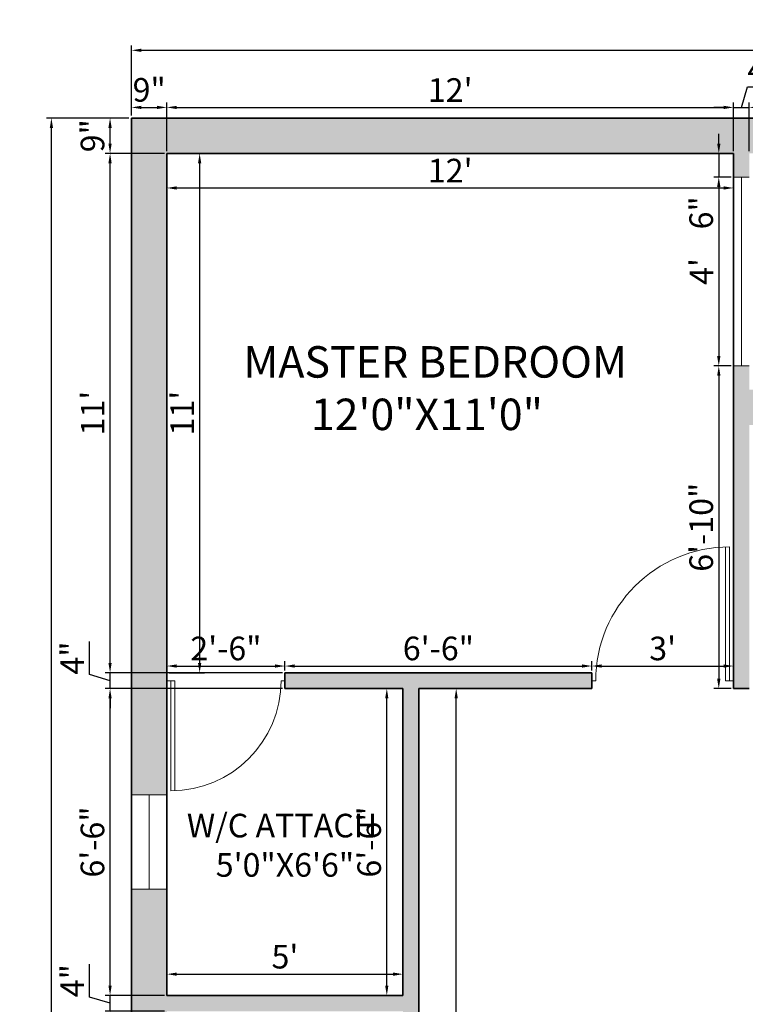
# Model space of a CAD drawing. Units: inches. Extents: x 3592 to 4861, y 1650 to 2243.
# Tile 29 of 30: x 4438 to 4622, y 1940 to 2190. Entities that reach past the tile are written whole.
import ezdxf

# ---------------------------------------------------------------- set-up
doc = ezdxf.new("R2010")
doc.units = ezdxf.units.IN
for name, color, linetype, lineweight in [('A-ANNO-DIMS', 2, 'Continuous', 13), ('A-AREA-IDEN', 7, 'Continuous', 18), ('A-DOOR', 3, 'Continuous', 20), ('A-GLAZ', 4, 'Continuous', 18), ('A-WALL', 7, 'Continuous', 35)]:
    doc.layers.add(name, color=color, linetype=linetype, lineweight=lineweight)
doc.layers.add('A-WALL-PATT', color=252, linetype='Continuous', lineweight=13, true_color=0x939598)
doc.styles.get("Standard").update_dxf_attribs({"font": 'arial.ttf'})
doc.dimstyles.new('ISO-25', dxfattribs={"dimtxt": 9, "dimasz": 2.5, "dimexe": 1.25, "dimexo": 0.625, "dimtad": 1, "dimlunit": 3, "dimtxsty": 'Standard', "dimcen": 2.5, "dimadec": 0, "dimazin": 0, "dimtfac": 1, "dimtmove": 0, "dimatfit": 3, "dimfxl": 1, "dimarcsym": 0})

# ---------------------------------------------------------------- blocks, each defined once
blk = doc.blocks.new('1')
for p, q in [((3628.27, 1890.86), (3628.27, 1924.86)), ((3629.27, 1890.86), (3629.27, 1924.86)), ((3627.27, 1890.86), (3629.27, 1890.86)), ((3662.27, 1890.86), (3663.27, 1890.86))]:
    blk.add_line(p, q)
blk.add_arc((3628.27, 1890.86), 34, 0, 90)
blk = doc.blocks.new('2')
for p, q in [((3637.19, 1914.49), (3637.19, 1942.49)), ((3638.19, 1914.49), (3638.19, 1942.49)), ((3636.19, 1914.49), (3638.19, 1914.49)), ((3665.19, 1914.49), (3666.19, 1914.49))]:
    blk.add_line(p, q)
blk.add_arc((3637.19, 1914.49), 28, 0, 90)
blk = doc.blocks.new('*D45')
at = {"layer": 'A-ANNO-DIMS', "color": 0, "lineweight": -2, "transparency": 16777216}
for p, q in [((4475.25, 2155.59), (4475.25, 2146.2)), ((4619.25, 2155.59), (4619.25, 2146.2)), ((4477.75, 2147.45), (4616.75, 2147.45))]:
    blk.add_line(p, q, dxfattribs=at)
at = {"layer": 'A-ANNO-DIMS', "color": 0, "transparency": 16777216}
for points in [[(4477.75, 2147.86), (4477.75, 2147.03), (4475.25, 2147.45)], [(4616.75, 2147.86), (4616.75, 2147.03), (4619.25, 2147.45)]]:
    blk.add_solid(points, dxfattribs=at)
at = {"layer": 'Defpoints', "color": 0, "transparency": 16777216}
for p in [(4475.25, 2156.22), (4619.25, 2156.22), (4619.25, 2147.45)]:
    blk.add_point(p, dxfattribs=at)
at = {"layer": 'A-ANNO-DIMS', "color": 0, "transparency": 16777216, "insert": (4547.25, 2151.08), "char_height": 6, "attachment_point": 5}
blk.add_mtext("12'", dxfattribs=at)
blk = doc.blocks.new('*D46')
at = {"layer": 'A-ANNO-DIMS', "color": 0, "lineweight": -2, "transparency": 16777216}
for p, q in [((4475.25, 2024.79), (4475.25, 2027.19)), ((4505.25, 2024.84), (4505.25, 2027.19)), ((4477.75, 2025.94), (4502.75, 2025.94))]:
    blk.add_line(p, q, dxfattribs=at)
at = {"layer": 'A-ANNO-DIMS', "color": 0, "transparency": 16777216}
for points in [[(4477.75, 2026.36), (4477.75, 2025.53), (4475.25, 2025.94)], [(4502.75, 2026.36), (4502.75, 2025.53), (4505.25, 2025.94)]]:
    blk.add_solid(points, dxfattribs=at)
at = {"layer": 'Defpoints', "color": 0, "transparency": 16777216}
for p in [(4505.25, 2025.94), (4475.25, 2024.17), (4505.25, 2024.22)]:
    blk.add_point(p, dxfattribs=at)
at = {"layer": 'A-ANNO-DIMS', "color": 0, "transparency": 16777216, "insert": (4490.25, 2029.63), "char_height": 6, "attachment_point": 5}
blk.add_mtext('2\'-6"', dxfattribs=at)
blk = doc.blocks.new('*D47')
at = {"layer": 'A-ANNO-DIMS', "color": 0, "lineweight": -2, "transparency": 16777216}
for p, q in [((4505.25, 2024.84), (4505.25, 2027.19)), ((4583.25, 2024.84), (4583.25, 2027.19)), ((4507.75, 2025.94), (4580.75, 2025.94))]:
    blk.add_line(p, q, dxfattribs=at)
at = {"layer": 'A-ANNO-DIMS', "color": 0, "transparency": 16777216}
for points in [[(4507.75, 2026.36), (4507.75, 2025.53), (4505.25, 2025.94)], [(4580.75, 2026.36), (4580.75, 2025.53), (4583.25, 2025.94)]]:
    blk.add_solid(points, dxfattribs=at)
at = {"layer": 'Defpoints', "color": 0, "transparency": 16777216}
for p in [(4583.25, 2025.94), (4505.25, 2024.22), (4583.25, 2024.22)]:
    blk.add_point(p, dxfattribs=at)
at = {"layer": 'A-ANNO-DIMS', "color": 0, "transparency": 16777216, "insert": (4544.25, 2029.63), "char_height": 6, "attachment_point": 5}
blk.add_mtext('6\'-6"', dxfattribs=at)
blk = doc.blocks.new('*D48')
at = {"layer": 'A-ANNO-DIMS', "color": 0, "lineweight": -2, "transparency": 16777216}
for p, q in [((4583.25, 2024.84), (4583.25, 2027.19)), ((4585.75, 2025.94), (4616.75, 2025.94)), ((4619.25, 2025.32), (4619.25, 2024.69))]:
    blk.add_line(p, q, dxfattribs=at)
at = {"layer": 'A-ANNO-DIMS', "color": 0, "transparency": 16777216}
for points in [[(4585.75, 2026.36), (4585.75, 2025.53), (4583.25, 2025.94)], [(4616.75, 2026.36), (4616.75, 2025.53), (4619.25, 2025.94)]]:
    blk.add_solid(points, dxfattribs=at)
at = {"layer": 'Defpoints', "color": 0, "transparency": 16777216}
for p in [(4619.25, 2025.94), (4619.25, 2025.94), (4583.25, 2024.22)]:
    blk.add_point(p, dxfattribs=at)
at = {"layer": 'A-ANNO-DIMS', "color": 0, "transparency": 16777216, "insert": (4601.25, 2029.63), "char_height": 6, "attachment_point": 5}
blk.add_mtext("3'", dxfattribs=at)
blk = doc.blocks.new('*D49')
at = {"layer": 'A-ANNO-DIMS', "color": 0, "lineweight": -2, "transparency": 16777216}
for p, q in [((4475.87, 2156.22), (4484.83, 2156.22)), ((4483.58, 2153.72), (4483.58, 2026.72)), ((4475.87, 2024.22), (4484.83, 2024.22))]:
    blk.add_line(p, q, dxfattribs=at)
at = {"layer": 'A-ANNO-DIMS', "color": 0, "transparency": 16777216}
for points in [[(4483.16, 2153.72), (4483.99, 2153.72), (4483.58, 2156.22)], [(4483.16, 2026.72), (4483.99, 2026.72), (4483.58, 2024.22)]]:
    blk.add_solid(points, dxfattribs=at)
at = {"layer": 'Defpoints', "color": 0, "transparency": 16777216}
for p in [(4475.25, 2156.22), (4475.25, 2024.22), (4483.58, 2024.22)]:
    blk.add_point(p, dxfattribs=at)
at = {"layer": 'A-ANNO-DIMS', "color": 0, "transparency": 16777216, "insert": (4479.94, 2090.22), "char_height": 6, "attachment_point": 5, "rotation": 90}
blk.add_mtext("11'", dxfattribs=at)
blk = doc.blocks.new('*D56')
at = {"layer": 'A-ANNO-DIMS', "color": 0, "lineweight": -2, "transparency": 16777216}
for p, q in [((4615.51, 2158.72), (4615.51, 2161.22)), ((4618.62, 2156.22), (4614.26, 2156.22)), ((4615.51, 2156.22), (4615.51, 2150.22)), ((4618.62, 2150.22), (4614.26, 2150.22)), ((4615.51, 2147.72), (4615.51, 2137.04))]:
    blk.add_line(p, q, dxfattribs=at)
at = {"layer": 'A-ANNO-DIMS', "color": 0, "transparency": 16777216}
for points in [[(4615.09, 2158.72), (4615.93, 2158.72), (4615.51, 2156.22)], [(4615.09, 2147.72), (4615.93, 2147.72), (4615.51, 2150.22)]]:
    blk.add_solid(points, dxfattribs=at)
at = {"layer": 'Defpoints', "color": 0, "transparency": 16777216}
for p in [(4619.25, 2156.22), (4615.51, 2150.22), (4619.25, 2150.22)]:
    blk.add_point(p, dxfattribs=at)
at = {"layer": 'A-ANNO-DIMS', "color": 0, "transparency": 16777216, "insert": (4611.82, 2141.13), "char_height": 6, "attachment_point": 5, "rotation": 90}
blk.add_mtext('6"', dxfattribs=at)
blk = doc.blocks.new('*D57')
at = {"layer": 'A-ANNO-DIMS', "color": 0, "lineweight": -2, "transparency": 16777216}
for p, q in [((4618.62, 2150.22), (4614.26, 2150.22)), ((4615.51, 2147.72), (4615.51, 2104.72)), ((4618.62, 2102.22), (4614.26, 2102.22))]:
    blk.add_line(p, q, dxfattribs=at)
at = {"layer": 'A-ANNO-DIMS', "color": 0, "transparency": 16777216}
for points in [[(4615.09, 2147.72), (4615.93, 2147.72), (4615.51, 2150.22)], [(4615.09, 2104.72), (4615.93, 2104.72), (4615.51, 2102.22)]]:
    blk.add_solid(points, dxfattribs=at)
at = {"layer": 'Defpoints', "color": 0, "transparency": 16777216}
for p in [(4619.25, 2150.22), (4615.51, 2102.22), (4619.25, 2102.22)]:
    blk.add_point(p, dxfattribs=at)
at = {"layer": 'A-ANNO-DIMS', "color": 0, "transparency": 16777216, "insert": (4611.88, 2126.22), "char_height": 6, "attachment_point": 5, "rotation": 90}
blk.add_mtext("4'", dxfattribs=at)
blk = doc.blocks.new('*D58')
at = {"layer": 'A-ANNO-DIMS', "color": 0, "lineweight": -2, "transparency": 16777216}
for p, q in [((4618.62, 2102.22), (4614.26, 2102.22)), ((4615.51, 2099.72), (4615.51, 2022.72)), ((4618.62, 2020.22), (4614.26, 2020.22))]:
    blk.add_line(p, q, dxfattribs=at)
at = {"layer": 'A-ANNO-DIMS', "color": 0, "transparency": 16777216}
for points in [[(4615.09, 2099.72), (4615.93, 2099.72), (4615.51, 2102.22)], [(4615.09, 2022.72), (4615.93, 2022.72), (4615.51, 2020.22)]]:
    blk.add_solid(points, dxfattribs=at)
at = {"layer": 'Defpoints', "color": 0, "transparency": 16777216}
for p in [(4619.25, 2102.22), (4615.51, 2020.22), (4619.25, 2020.22)]:
    blk.add_point(p, dxfattribs=at)
at = {"layer": 'A-ANNO-DIMS', "color": 0, "transparency": 16777216, "insert": (4611.82, 2061.22), "char_height": 6, "attachment_point": 5, "rotation": 90}
blk.add_mtext('6\'-10"', dxfattribs=at)
blk = doc.blocks.new('*D90')
at = {"layer": 'A-ANNO-DIMS', "color": 0, "lineweight": -2, "transparency": 16777216}
for p, q in [((4475.25, 1942.84), (4475.25, 1948.88)), ((4477.75, 1947.63), (4532.75, 1947.63)), ((4535.25, 1942.84), (4535.25, 1948.88))]:
    blk.add_line(p, q, dxfattribs=at)
at = {"layer": 'A-ANNO-DIMS', "color": 0, "transparency": 16777216}
for points in [[(4477.75, 1948.04), (4477.75, 1947.21), (4475.25, 1947.63)], [(4532.75, 1948.04), (4532.75, 1947.21), (4535.25, 1947.63)]]:
    blk.add_solid(points, dxfattribs=at)
at = {"layer": 'Defpoints', "color": 0, "transparency": 16777216}
for p in [(4535.25, 1947.63), (4475.25, 1942.22), (4535.25, 1942.22)]:
    blk.add_point(p, dxfattribs=at)
at = {"layer": 'A-ANNO-DIMS', "color": 0, "transparency": 16777216, "insert": (4505.25, 1951.3), "char_height": 6, "attachment_point": 5}
blk.add_mtext("5'", dxfattribs=at)
blk = doc.blocks.new('*D91')
at = {"layer": 'A-ANNO-DIMS', "color": 0, "lineweight": -2, "transparency": 16777216}
for p, q in [((4534.62, 2020.22), (4529.89, 2020.22)), ((4531.14, 1944.72), (4531.14, 2017.72)), ((4534.62, 1942.22), (4529.89, 1942.22))]:
    blk.add_line(p, q, dxfattribs=at)
at = {"layer": 'A-ANNO-DIMS', "color": 0, "transparency": 16777216}
for points in [[(4530.72, 2017.72), (4531.55, 2017.72), (4531.14, 2020.22)], [(4530.72, 1944.72), (4531.55, 1944.72), (4531.14, 1942.22)]]:
    blk.add_solid(points, dxfattribs=at)
at = {"layer": 'Defpoints', "color": 0, "transparency": 16777216}
for p in [(4531.14, 2020.22), (4535.25, 2020.22), (4535.25, 1942.22)]:
    blk.add_point(p, dxfattribs=at)
at = {"layer": 'A-ANNO-DIMS', "color": 0, "transparency": 16777216, "insert": (4527.45, 1981.22), "char_height": 6, "attachment_point": 5, "rotation": 90}
blk.add_mtext('6\'-6"', dxfattribs=at)
blk = doc.blocks.new('*D92')
at = {"layer": 'A-ANNO-DIMS', "color": 0, "lineweight": -2, "transparency": 16777216}
for p, q in [((4546.11, 2020.22), (4550.03, 2020.22)), ((4548.78, 1819.72), (4548.78, 2017.72)), ((4546.11, 1817.22), (4550.03, 1817.22))]:
    blk.add_line(p, q, dxfattribs=at)
at = {"layer": 'A-ANNO-DIMS', "color": 0, "transparency": 16777216}
for points in [[(4548.36, 2017.72), (4549.19, 2017.72), (4548.78, 2020.22)], [(4548.36, 1819.72), (4549.19, 1819.72), (4548.78, 1817.22)]]:
    blk.add_solid(points, dxfattribs=at)
at = {"layer": 'Defpoints', "color": 0, "transparency": 16777216}
for p in [(4545.48, 2020.22), (4548.78, 2020.22), (4545.48, 1817.22)]:
    blk.add_point(p, dxfattribs=at)
at = {"layer": 'A-ANNO-DIMS', "color": 0, "transparency": 16777216, "insert": (4545.09, 1918.72), "char_height": 6, "attachment_point": 5, "rotation": 90}
blk.add_mtext('16\'-11"', dxfattribs=at)
blk = doc.blocks.new('*D106')
at = {"layer": 'A-ANNO-DIMS', "color": 0, "lineweight": -2, "transparency": 16777216}
for p, q in [((4455.62, 1941.78), (4455.62, 1950.16)), ((4460.81, 1944.72), (4460.81, 1947.22)), ((4474.62, 1942.22), (4459.56, 1942.22)), ((4460.81, 1938.22), (4460.81, 1942.22)), ((4460.81, 1938.22), (4460.81, 1942.22)), ((4460.81, 1940.22), (4455.62, 1941.78)), ((4474.62, 1938.22), (4459.56, 1938.22)), ((4460.81, 1935.72), (4460.81, 1933.22))]:
    blk.add_line(p, q, dxfattribs=at)
at = {"layer": 'A-ANNO-DIMS', "color": 0, "transparency": 16777216}
for points in [[(4460.39, 1944.72), (4461.22, 1944.72), (4460.81, 1942.22)], [(4460.39, 1935.72), (4461.22, 1935.72), (4460.81, 1938.22)]]:
    blk.add_solid(points, dxfattribs=at)
at = {"layer": 'Defpoints', "color": 0, "transparency": 16777216}
for p in [(4460.81, 1942.22), (4475.25, 1942.22), (4475.25, 1938.22)]:
    blk.add_point(p, dxfattribs=at)
at = {"layer": 'A-ANNO-DIMS', "color": 0, "transparency": 16777216, "insert": (4451.99, 1945.97), "char_height": 6, "attachment_point": 5, "rotation": 90}
blk.add_mtext('4"', dxfattribs=at)
blk = doc.blocks.new('*D107')
at = {"layer": 'A-ANNO-DIMS', "color": 0, "lineweight": -2, "transparency": 16777216}
for p, q in [((4504.62, 2020.22), (4459.56, 2020.22)), ((4460.81, 1944.72), (4460.81, 2017.72)), ((4474.62, 1942.22), (4459.56, 1942.22))]:
    blk.add_line(p, q, dxfattribs=at)
at = {"layer": 'A-ANNO-DIMS', "color": 0, "transparency": 16777216}
for points in [[(4460.39, 2017.72), (4461.22, 2017.72), (4460.81, 2020.22)], [(4460.39, 1944.72), (4461.22, 1944.72), (4460.81, 1942.22)]]:
    blk.add_solid(points, dxfattribs=at)
at = {"layer": 'Defpoints', "color": 0, "transparency": 16777216}
for p in [(4460.81, 2020.22), (4505.25, 2020.22), (4475.25, 1942.22)]:
    blk.add_point(p, dxfattribs=at)
at = {"layer": 'A-ANNO-DIMS', "color": 0, "transparency": 16777216, "insert": (4457.12, 1981.22), "char_height": 6, "attachment_point": 5, "rotation": 90}
blk.add_mtext('6\'-6"', dxfattribs=at)
blk = doc.blocks.new('*D108')
at = {"layer": 'A-ANNO-DIMS', "color": 0, "lineweight": -2, "transparency": 16777216}
for p, q in [((4455.62, 2023.78), (4455.62, 2032.16)), ((4460.81, 2026.72), (4460.81, 2029.22)), ((4460.81, 2022.22), (4455.62, 2023.78)), ((4504.62, 2024.22), (4459.56, 2024.22)), ((4460.81, 2020.22), (4460.81, 2024.22)), ((4460.81, 2020.22), (4460.81, 2024.22)), ((4504.62, 2020.22), (4459.56, 2020.22)), ((4460.81, 2017.72), (4460.81, 2015.22))]:
    blk.add_line(p, q, dxfattribs=at)
at = {"layer": 'A-ANNO-DIMS', "color": 0, "transparency": 16777216}
for points in [[(4460.39, 2026.72), (4461.22, 2026.72), (4460.81, 2024.22)], [(4460.39, 2017.72), (4461.22, 2017.72), (4460.81, 2020.22)]]:
    blk.add_solid(points, dxfattribs=at)
at = {"layer": 'Defpoints', "color": 0, "transparency": 16777216}
for p in [(4460.81, 2024.22), (4505.25, 2024.22), (4505.25, 2020.22)]:
    blk.add_point(p, dxfattribs=at)
at = {"layer": 'A-ANNO-DIMS', "color": 0, "transparency": 16777216, "insert": (4451.99, 2027.97), "char_height": 6, "attachment_point": 5, "rotation": 90}
blk.add_mtext('4"', dxfattribs=at)
blk = doc.blocks.new('*D109')
at = {"layer": 'A-ANNO-DIMS', "color": 0, "lineweight": -2, "transparency": 16777216}
for p, q in [((4474.62, 2156.22), (4459.56, 2156.22)), ((4460.81, 2026.72), (4460.81, 2153.72)), ((4504.62, 2024.22), (4459.56, 2024.22))]:
    blk.add_line(p, q, dxfattribs=at)
at = {"layer": 'A-ANNO-DIMS', "color": 0, "transparency": 16777216}
for points in [[(4460.39, 2153.72), (4461.22, 2153.72), (4460.81, 2156.22)], [(4460.39, 2026.72), (4461.22, 2026.72), (4460.81, 2024.22)]]:
    blk.add_solid(points, dxfattribs=at)
at = {"layer": 'Defpoints', "color": 0, "transparency": 16777216}
for p in [(4460.81, 2156.22), (4475.25, 2156.22), (4505.25, 2024.22)]:
    blk.add_point(p, dxfattribs=at)
at = {"layer": 'A-ANNO-DIMS', "color": 0, "transparency": 16777216, "insert": (4457.17, 2090.22), "char_height": 6, "attachment_point": 5, "rotation": 90}
blk.add_mtext("11'", dxfattribs=at)
blk = doc.blocks.new('*D110')
at = {"layer": 'A-ANNO-DIMS', "color": 0, "lineweight": -2, "transparency": 16777216}
for p, q in [((4465.62, 2165.22), (4459.56, 2165.22)), ((4460.81, 2158.72), (4460.81, 2162.72)), ((4474.62, 2156.22), (4459.56, 2156.22))]:
    blk.add_line(p, q, dxfattribs=at)
at = {"layer": 'A-ANNO-DIMS', "color": 0, "transparency": 16777216}
for points in [[(4460.39, 2162.72), (4461.22, 2162.72), (4460.81, 2165.22)], [(4460.39, 2158.72), (4461.22, 2158.72), (4460.81, 2156.22)]]:
    blk.add_solid(points, dxfattribs=at)
at = {"layer": 'Defpoints', "color": 0, "transparency": 16777216}
for p in [(4460.81, 2165.22), (4466.25, 2165.22), (4475.25, 2156.22)]:
    blk.add_point(p, dxfattribs=at)
at = {"layer": 'A-ANNO-DIMS', "color": 0, "transparency": 16777216, "insert": (4457.12, 2160.72), "char_height": 6, "attachment_point": 5, "rotation": 90}
blk.add_mtext('9"', dxfattribs=at)
blk = doc.blocks.new('*D111')
at = {"layer": 'A-ANNO-DIMS', "color": 0, "lineweight": -2, "transparency": 16777216}
for p, q in [((4466.25, 2165.84), (4466.25, 2169.17)), ((4468.75, 2167.92), (4472.75, 2167.92)), ((4475.25, 2156.84), (4475.25, 2169.17))]:
    blk.add_line(p, q, dxfattribs=at)
at = {"layer": 'A-ANNO-DIMS', "color": 0, "transparency": 16777216}
for points in [[(4468.75, 2168.33), (4468.75, 2167.5), (4466.25, 2167.92)], [(4472.75, 2168.33), (4472.75, 2167.5), (4475.25, 2167.92)]]:
    blk.add_solid(points, dxfattribs=at)
at = {"layer": 'Defpoints', "color": 0, "transparency": 16777216}
for p in [(4475.25, 2167.92), (4466.25, 2165.22), (4475.25, 2156.22)]:
    blk.add_point(p, dxfattribs=at)
at = {"layer": 'A-ANNO-DIMS', "color": 0, "transparency": 16777216, "insert": (4470.75, 2171.61), "char_height": 6, "attachment_point": 5}
blk.add_mtext('9"', dxfattribs=at)
blk = doc.blocks.new('*D112')
at = {"layer": 'A-ANNO-DIMS', "color": 0, "lineweight": -2, "transparency": 16777216}
for p, q in [((4475.25, 2156.84), (4475.25, 2169.17)), ((4477.75, 2167.92), (4616.75, 2167.92)), ((4619.25, 2156.84), (4619.25, 2169.17))]:
    blk.add_line(p, q, dxfattribs=at)
at = {"layer": 'A-ANNO-DIMS', "color": 0, "transparency": 16777216}
for points in [[(4477.75, 2168.33), (4477.75, 2167.5), (4475.25, 2167.92)], [(4616.75, 2168.33), (4616.75, 2167.5), (4619.25, 2167.92)]]:
    blk.add_solid(points, dxfattribs=at)
at = {"layer": 'Defpoints', "color": 0, "transparency": 16777216}
for p in [(4619.25, 2167.92), (4475.25, 2156.22), (4619.25, 2156.22)]:
    blk.add_point(p, dxfattribs=at)
at = {"layer": 'A-ANNO-DIMS', "color": 0, "transparency": 16777216, "insert": (4547.25, 2171.56), "char_height": 6, "attachment_point": 5}
blk.add_mtext("12'", dxfattribs=at)
blk = doc.blocks.new('*D113')
at = {"layer": 'A-ANNO-DIMS', "color": 0, "lineweight": -2, "transparency": 16777216}
for p, q in [((4621.25, 2167.92), (4622.81, 2173.11)), ((4622.81, 2173.11), (4631.19, 2173.11)), ((4616.75, 2167.92), (4614.25, 2167.92)), ((4619.25, 2156.84), (4619.25, 2169.17)), ((4619.25, 2167.92), (4623.25, 2167.92)), ((4619.25, 2167.92), (4623.25, 2167.92)), ((4623.25, 2156.84), (4623.25, 2169.17)), ((4625.75, 2167.92), (4628.25, 2167.92))]:
    blk.add_line(p, q, dxfattribs=at)
at = {"layer": 'A-ANNO-DIMS', "color": 0, "transparency": 16777216}
for points in [[(4616.75, 2168.33), (4616.75, 2167.5), (4619.25, 2167.92)], [(4625.75, 2168.33), (4625.75, 2167.5), (4623.25, 2167.92)]]:
    blk.add_solid(points, dxfattribs=at)
at = {"layer": 'Defpoints', "color": 0, "transparency": 16777216}
for p in [(4623.25, 2167.92), (4619.25, 2156.22), (4623.25, 2156.22)]:
    blk.add_point(p, dxfattribs=at)
at = {"layer": 'A-ANNO-DIMS', "color": 0, "transparency": 16777216, "insert": (4627, 2176.73), "char_height": 6, "attachment_point": 5}
blk.add_mtext('4"', dxfattribs=at)
blk = doc.blocks.new('*D131')
at = {"layer": 'A-ANNO-DIMS', "color": 0, "lineweight": -2, "transparency": 16777216}
for p, q in [((4465.62, 2165.22), (4444.65, 2165.22)), ((4445.9, 1687.72), (4445.9, 2162.72)), ((4465.62, 1685.22), (4444.65, 1685.22))]:
    blk.add_line(p, q, dxfattribs=at)
at = {"layer": 'A-ANNO-DIMS', "color": 0, "transparency": 16777216}
for points in [[(4445.49, 2162.72), (4446.32, 2162.72), (4445.9, 2165.22)], [(4445.49, 1687.72), (4446.32, 1687.72), (4445.9, 1685.22)]]:
    blk.add_solid(points, dxfattribs=at)
at = {"layer": 'Defpoints', "color": 0, "transparency": 16777216}
for p in [(4445.9, 2165.22), (4466.25, 2165.22), (4466.25, 1685.22)]:
    blk.add_point(p, dxfattribs=at)
at = {"layer": 'A-ANNO-DIMS', "color": 0, "transparency": 16777216, "insert": (4442.21, 1925.22), "char_height": 6, "attachment_point": 5, "rotation": 90}
blk.add_mtext("40'", dxfattribs=at)
blk = doc.blocks.new('*D132')
at = {"layer": 'A-ANNO-DIMS', "color": 0, "lineweight": -2, "transparency": 16777216}
for p, q in [((4466.25, 2165.84), (4466.25, 2183.69)), ((4468.75, 2182.44), (4823.75, 2182.44)), ((4826.25, 2165.84), (4826.25, 2183.69))]:
    blk.add_line(p, q, dxfattribs=at)
at = {"layer": 'A-ANNO-DIMS', "color": 0, "transparency": 16777216}
for points in [[(4468.75, 2182.85), (4468.75, 2182.02), (4466.25, 2182.44)], [(4823.75, 2182.85), (4823.75, 2182.02), (4826.25, 2182.44)]]:
    blk.add_solid(points, dxfattribs=at)
at = {"layer": 'Defpoints', "color": 0, "transparency": 16777216}
for p in [(4826.25, 2182.44), (4466.25, 2165.22), (4826.25, 2165.22)]:
    blk.add_point(p, dxfattribs=at)
at = {"layer": 'A-ANNO-DIMS', "color": 0, "transparency": 16777216, "insert": (4646.25, 2186.13), "char_height": 6, "attachment_point": 5}
blk.add_mtext("30'", dxfattribs=at)
blk = doc.blocks.new('*D158')
at = {"layer": 'A-ANNO-DIMS', "color": 0, "lineweight": -2, "transparency": 16777216}
for p, q in [((4281.9, 1934.46), (4281.9, 1921.52)), ((4364, 1934.46), (4364, 1921.52)), ((4284.4, 1922.77), (4361.5, 1922.77)), ((4364, 1922.77), (4473.66, 1922.77))]:
    blk.add_line(p, q, dxfattribs=at)
at = {"layer": 'A-ANNO-DIMS', "color": 0, "transparency": 16777216}
for points in [[(4284.4, 1923.19), (4284.4, 1922.36), (4281.9, 1922.77)], [(4361.5, 1923.19), (4361.5, 1922.36), (4364, 1922.77)]]:
    blk.add_solid(points, dxfattribs=at)
at = {"layer": 'Defpoints', "color": 0, "transparency": 16777216}
for p in [(4281.9, 1935.09), (4364, 1935.09), (4364, 1922.77)]:
    blk.add_point(p, dxfattribs=at)
at = {"layer": 'A-ANNO-DIMS', "color": 0, "transparency": 16777216, "insert": (4420.08, 1928.05), "char_height": 9, "attachment_point": 5}
blk.add_mtext('DINING SET 6\'-10"', dxfattribs=at)

msp = doc.modelspace()

# ---------------------------------------------------------------- hatches: boundary and pattern name
at = {"layer": 'A-WALL-PATT'}
h = msp.add_hatch(color=256, dxfattribs=at)
h.dxf.hatch_style = 1
h.paths.add_polyline_path([(4466.25, 2165.219), (4466.25, 1993.219), (4475.25, 1993.219), (4475.25, 2156.219), (4619.25, 2156.219), (4619.25, 2150.219), (4623.25, 2150.219), (4623.25, 2156.219), (4684.25, 2156.219), (4684.25, 2150.219), (4693.25, 2150.219), (4693.25, 2156.219), (4817.25, 2156.219), (4817.25, 2114.219), (4826.25, 2114.219), (4826.25, 2165.219)])
h.paths.add_polyline_path([(4623.25, 2096.219), (4623.25, 2102.219), (4619.25, 2102.219), (4619.25, 2020.219), (4623.25, 2020.219), (4623.25, 2087.219), (4684.25, 2087.219), (4684.25, 2020.219), (4734.25, 2020.219), (4734.25, 2024.219), (4693.25, 2024.219), (4693.25, 2102.219), (4684.25, 2102.219), (4684.25, 2096.219)], flags=17)
h.paths.add_polyline_path([(4817.25, 2024.219), (4776.25, 2024.219), (4776.25, 2020.219), (4817.25, 2020.219), (4817.25, 1989.719), (4826.25, 1989.719), (4826.25, 2066.219), (4817.25, 2066.219)])
h.paths.add_polyline_path([(4817.25, 1865.219), (4826.25, 1865.219), (4826.25, 1941.719), (4817.25, 1941.719), (4817.25, 1911.219), (4729.25, 1911.219), (4729.25, 1907.219), (4817.25, 1907.219)])
h.paths.add_polyline_path([(4826.25, 1817.219), (4817.25, 1817.219), (4817.25, 1775.219), (4693.25, 1775.219), (4693.25, 1911.219), (4684.25, 1911.219), (4684.25, 1817.219), (4648.75, 1817.219), (4648.75, 1808.219), (4684.25, 1808.219), (4684.25, 1766.219), (4817.25, 1766.219), (4817.25, 1694.219), (4684.25, 1694.219), (4684.25, 1685.219), (4826.25, 1685.219)])
h.paths.add_polyline_path([(4505.25, 1817.219), (4505.25, 1808.219), (4606.75, 1808.219), (4606.75, 1817.219)])
h.paths.add_polyline_path([(4539.25, 1856.219), (4539.25, 2020.219), (4583.25, 2020.219), (4583.25, 2024.219), (4505.25, 2024.219), (4505.25, 2020.219), (4535.25, 2020.219), (4535.25, 1942.219), (4475.25, 1942.219), (4475.25, 1969.219), (4466.25, 1969.219), (4466.25, 1911.219), (4475.25, 1911.219), (4475.25, 1938.219), (4535.25, 1938.219), (4535.25, 1860.219), (4505.25, 1860.219), (4505.25, 1856.219)])
h.paths.add_polyline_path([(4475.25, 1887.219), (4466.25, 1887.219), (4466.25, 1685.219), (4580.25, 1685.219), (4580.25, 1715.219), (4571.25, 1715.219), (4571.25, 1694.219), (4475.25, 1694.219)])
h.paths.add_polyline_path([(4571.25, 1751.219), (4580.25, 1751.219), (4580.25, 1772.219), (4571.25, 1772.219)], flags=17)

# ---------------------------------------------------------------- linework, layer by layer
at = {"layer": 'A-GLAZ'}
for p, q in [((4623.25, 2150.219), (4619.25, 2150.219)), ((4621.25, 2150.219), (4621.25, 2102.219)), ((4623.25, 2102.219), (4619.25, 2102.219)), ((4475.25, 1993.219), (4466.25, 1993.219)), ((4470.75, 1993.219), (4470.75, 1969.219)), ((4475.25, 1969.219), (4466.25, 1969.219))]:
    msp.add_line(p, q, dxfattribs=at)
at = {"layer": 'A-WALL'}
for p, q in [((4466.25, 2165.219), (4826.25, 2165.219)), ((4466.25, 1685.219), (4466.25, 2165.219)), ((4475.25, 2156.219), (4619.25, 2156.219)), ((4475.25, 1942.219), (4475.25, 2156.219)), ((4619.25, 2020.219), (4619.25, 2156.219)), ((4505.25, 2024.219), (4583.25, 2024.219)), ((4505.25, 2020.219), (4505.25, 2024.219)), ((4583.25, 2020.219), (4583.25, 2024.219)), ((4505.25, 2020.219), (4535.25, 2020.219)), ((4535.25, 1942.219), (4535.25, 2020.219)), ((4539.25, 2020.219), (4583.25, 2020.219)), ((4539.25, 1856.219), (4539.25, 2020.219)), ((4619.25, 2020.219), (4623.25, 2020.219)), ((4475.25, 1942.219), (4535.25, 1942.219))]:
    msp.add_line(p, q, dxfattribs=at)

# ---------------------------------------------------------------- block references
at = {"layer": 'A-DOOR', "xscale": -1}
msp.add_blockref('1', (8246.517, 131.354), dxfattribs=at)
at = {"layer": 'A-DOOR', "xscale": -1, "rotation": 180}
msp.add_blockref('2', (839.061, 3936.711), dxfattribs=at)

# ---------------------------------------------------------------- texts
at = {"layer": 'A-AREA-IDEN', "attachment_point": 1}
for s, insert, char_height in [('MASTER BEDROOM\\P       12\'0"X11\'0"', (4494.71, 2107.241), 8), ('W/C ATTACH\\P    5\'0"X6\'6"', (4480.334, 1988.392), 6)]:
    msp.add_mtext_dynamic_manual_height_columns(s, width=121.44943, gutter_width=12.5, heights=[0], dxfattribs=dict(at, insert=insert, char_height=char_height))

# ---------------------------------------------------------------- dimensions: what is measured, and where the dimension line sits
at = {"layer": 'A-ANNO-DIMS'}
for base, p1, p2, override, picture, middle in [((4826.25, 2182.436), (4466.25, 2165.219), (4826.25, 2165.219), {"dimtxt": 6, "dimclrd": 0, "dimclre": 0, "dimclrt": 0}, '*D132', (4646.25, 2186.127)), ((4623.25, 2167.918), (4619.25, 2156.219), (4623.25, 2156.219), {"dimtxt": 6, "dimclrd": 0, "dimclre": 0, "dimclrt": 0, "dimtmove": 1}, '*D113', (4623.431, 2176.73)), ((4475.25, 2167.918), (4466.25, 2165.219), (4475.25, 2156.219), {"dimtxt": 6, "dimclrd": 0, "dimclre": 0, "dimclrt": 0}, '*D111', (4470.75, 2171.606)), ((4619.25, 2167.918), (4475.25, 2156.219), (4619.25, 2156.219), {"dimtxt": 6, "dimclrd": 0, "dimclre": 0, "dimclrt": 0, "dimtmove": 1}, '*D112', (4547.25, 2171.555)), ((4619.25, 2147.447), (4475.25, 2156.219), (4619.25, 2156.219), {"dimtxt": 6, "dimclrd": 0, "dimclre": 0, "dimclrt": 0}, '*D45', (4547.25, 2151.084)), ((4505.25, 2025.942), (4475.25, 2024.165), (4505.25, 2024.219), {"dimtxt": 6, "dimclrd": 0, "dimclre": 0, "dimclrt": 0}, '*D46', (4490.25, 2029.631)), ((4583.25, 2025.942), (4505.25, 2024.219), (4583.25, 2024.219), {"dimtxt": 6, "dimclrd": 0, "dimclre": 0, "dimclrt": 0, "dimtmove": 1}, '*D47', (4544.25, 2029.631)), ((4619.25, 2025.942), (4583.25, 2024.219), (4619.25, 2025.942), {"dimtxt": 6, "dimclrd": 0, "dimclre": 0, "dimclrt": 0, "dimtmove": 1}, '*D48', (4601.25, 2029.633)), ((4535.25, 1947.627), (4475.25, 1942.219), (4535.25, 1942.219), {"dimtxt": 6, "dimclrd": 0, "dimclre": 0, "dimclrt": 0}, '*D90', (4505.25, 1951.303))]:
    dim = msp.add_linear_dim(base=base, p1=p1, p2=p2, dimstyle='ISO-25', override=override, dxfattribs=at)
    dim.commit()
    dim.dimension.update_dxf_attribs({"geometry": picture, "text_midpoint": middle})
for base, p1, p2, override, picture, middle in [((4445.902, 2165.219), (4466.25, 1685.219), (4466.25, 2165.219), {"dimtxt": 6, "dimclrd": 0, "dimclre": 0, "dimclrt": 0}, '*D131', (4442.214, 1925.219)), ((4460.807, 2165.219), (4475.25, 2156.219), (4466.25, 2165.219), {"dimtxt": 6, "dimclrd": 0, "dimclre": 0, "dimclrt": 0, "dimtmove": 1}, '*D110', (4457.118, 2160.719)), ((4615.509, 2150.219), (4619.25, 2156.219), (4619.25, 2150.219), {"dimtxt": 6, "dimclrd": 0, "dimclre": 0, "dimclrt": 0}, '*D56', (4611.821, 2141.129)), ((4460.807, 2156.219), (4505.25, 2024.219), (4475.25, 2156.219), {"dimtxt": 6, "dimclrd": 0, "dimclre": 0, "dimclrt": 0, "dimtmove": 1}, '*D109', (4457.17, 2090.219)), ((4483.576, 2024.219), (4475.25, 2156.219), (4475.25, 2024.219), {"dimtxt": 6, "dimclrd": 0, "dimclre": 0, "dimclrt": 0}, '*D49', (4479.939, 2090.219)), ((4615.509, 2102.219), (4619.25, 2150.219), (4619.25, 2102.219), {"dimtxt": 6, "dimclrd": 0, "dimclre": 0, "dimclrt": 0, "dimtmove": 1}, '*D57', (4611.884, 2126.219)), ((4615.509, 2020.219), (4619.25, 2102.219), (4619.25, 2020.219), {"dimtxt": 6, "dimclrd": 0, "dimclre": 0, "dimclrt": 0, "dimtmove": 1}, '*D58', (4611.821, 2061.219)), ((4460.807, 2024.219), (4505.25, 2020.219), (4505.25, 2024.219), {"dimtxt": 6, "dimclrd": 0, "dimclre": 0, "dimclrt": 0, "dimtmove": 1}, '*D108', (4451.994, 2024.4)), ((4460.807, 2020.219), (4475.25, 1942.219), (4505.25, 2020.219), {"dimtxt": 6, "dimclrd": 0, "dimclre": 0, "dimclrt": 0, "dimtmove": 1}, '*D107', (4457.118, 1981.219)), ((4531.138, 2020.219), (4535.25, 1942.219), (4535.25, 2020.219), {"dimtxt": 6, "dimclrd": 0, "dimclre": 0, "dimclrt": 0}, '*D91', (4527.449, 1981.219)), ((4548.776, 2020.219), (4545.484, 1817.219), (4545.484, 2020.219), {"dimtxt": 6, "dimclrd": 0, "dimclre": 0, "dimclrt": 0}, '*D92', (4545.088, 1918.719)), ((4460.807, 1942.219), (4475.25, 1938.219), (4475.25, 1942.219), {"dimtxt": 6, "dimclrd": 0, "dimclre": 0, "dimclrt": 0, "dimtmove": 1}, '*D106', (4451.994, 1942.4))]:
    dim = msp.add_linear_dim(base=base, p1=p1, p2=p2, angle=90, dimstyle='ISO-25', override=override, dxfattribs=at)
    dim.commit()
    dim.dimension.update_dxf_attribs({"geometry": picture, "text_midpoint": middle})
dim = msp.add_linear_dim(base=(4363.996, 1922.774), p1=(4281.898, 1935.089), p2=(4363.996, 1935.089), text='DINING SET <>', dimstyle='ISO-25', override={"dimdec": 1, "dimlfac": 1, "dimrnd": 0, "dimzin": 1, "dimdsep": 46, "dimlunit": 4, "dimfrac": 2}, dxfattribs=at)
dim.commit()
dim.dimension.update_dxf_attribs({"geometry": '*D158', "text_midpoint": (4420.077, 1928.052)})

doc.saveas('drawing.dxf')
